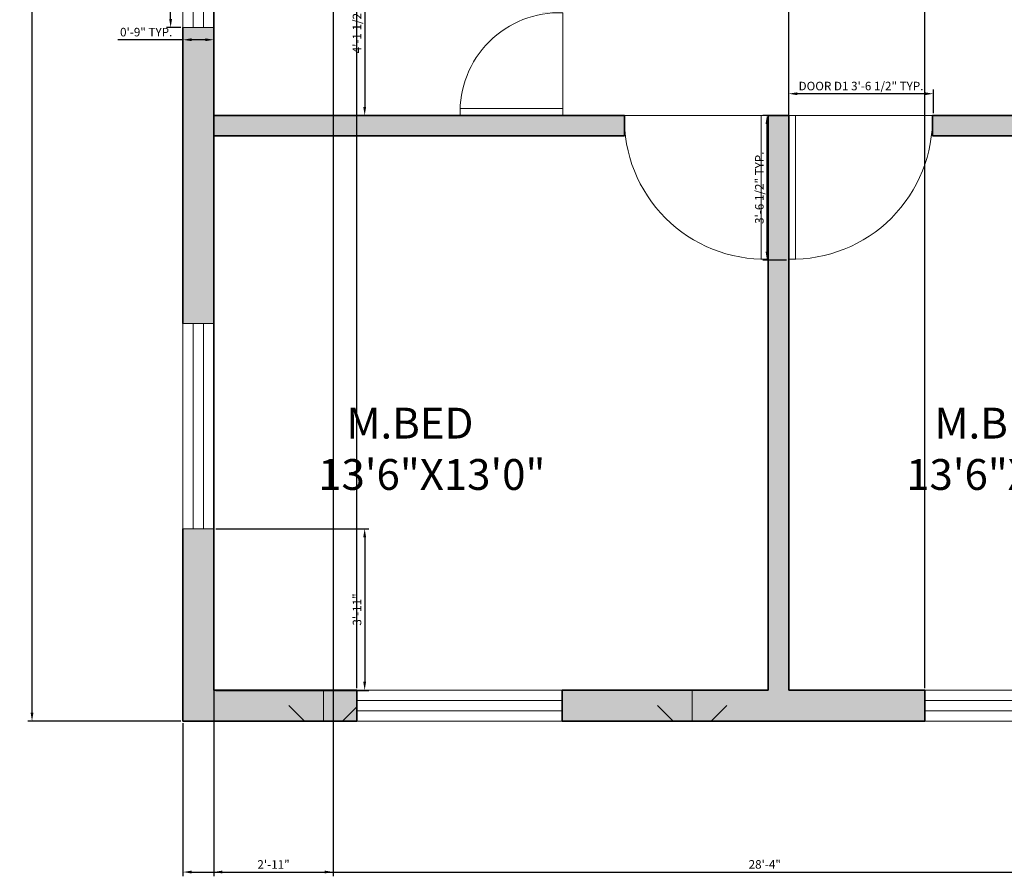
# Model space of a CAD drawing. Units: inches. Extents: x 1851 to 3979, y 3948 to 8145.
# Tile 1 of 4: x 1851 to 2139, y 3948 to 4198. Entities that reach past the tile are written whole.
import ezdxf

# ---------------------------------------------------------------- set-up
doc = ezdxf.new("R2010")
doc.units = ezdxf.units.IN
for name, color, linetype, lineweight in [('A-ANNO-DIMS', 2, 'Continuous', 18), ('A-GLAZ', 140, 'Continuous', 18), ('A-WALL', 7, 'Continuous', 35)]:
    doc.layers.add(name, color=color, linetype=linetype, lineweight=lineweight)
for name, color, linetype, lineweight, true_color in [('A-AREA-IDEN', 9, 'Continuous', 18, 0xc7c8ca), ('A-DOOR', 52, 'Continuous', 18, 0xc8c92d), ('A-WALL-PATT', 159, 'Continuous', 13, 0x22346e)]:
    doc.layers.add(name, color=color, linetype=linetype, lineweight=lineweight, true_color=true_color)
doc.styles.get("Standard").update_dxf_attribs({"font": 'arial.ttf'})
doc.dimstyles.new('ISO-25', dxfattribs={"dimtxt": 2.5, "dimasz": 2.5, "dimexe": 1.25, "dimexo": 0.625, "dimtad": 1, "dimlunit": 3, "dimtxsty": 'Standard', "dimcen": 2.5, "dimadec": 0, "dimazin": 0, "dimtfac": 1, "dimtmove": 0, "dimatfit": 3, "dimfxl": 1, "dimarcsym": 0})

# ---------------------------------------------------------------- blocks, each defined once
blk = doc.blocks.new('DOOR-SINGLE-42IN')
for p, q in [((42, 42), (40, 42)), ((40, 42), (40, 0)), ((42, 0), (42, 42)), ((40, 0), (42, 0))]:
    blk.add_line(p, q)
blk.add_arc((41, 1), 41.01, 88.6028, 181.3972)
blk = doc.blocks.new('DOOR-SINGLE-30IN')
for p, q in [((30, 2), (0, 2)), ((0, 2), (0, 0)), ((0, 0), (30, 0)), ((30, 0), (30, 2))]:
    blk.add_line(p, q)
blk.add_arc((1, 1), 29.02, 358.0251, 91.9749)
blk = doc.blocks.new('WINDOW-60IN')
for p, q in [((0, 9), (60, 9)), ((0, 0), (0, 9)), ((60, 9), (60, 0)), ((0, 6), (60, 6)), ((0, 3), (60, 3)), ((60, 0), (0, 0))]:
    blk.add_line(p, q)
blk = doc.blocks.new('WINDOW-24IN')
for p, q in [((0, 0), (0, 9)), ((0, 9), (24, 9)), ((24, 9), (24, 0)), ((0, 6), (24, 6)), ((0, 3), (24, 3)), ((24, 0), (0, 0))]:
    blk.add_line(p, q)
blk = doc.blocks.new('*D12')
at = {"layer": 'A-ANNO-DIMS', "color": 0, "lineweight": -2, "transparency": 16777216}
for p, q in [((1895.14, 4219.57), (1895.14, 4261.17)), ((1898.11, 4219.57), (1893.89, 4219.57)), ((1895.14, 4198.07), (1895.14, 4217.07)), ((1898.11, 4195.57), (1893.89, 4195.57))]:
    blk.add_line(p, q, dxfattribs=at)
at = {"layer": 'A-ANNO-DIMS', "color": 0, "transparency": 16777216}
for points in [[(1894.72, 4217.07), (1895.55, 4217.07), (1895.14, 4219.57)], [(1894.72, 4198.07), (1895.55, 4198.07), (1895.14, 4195.57)]]:
    blk.add_solid(points, dxfattribs=at)
at = {"layer": 'Defpoints', "color": 0, "transparency": 16777216}
for p in [(1895.14, 4219.57), (1898.74, 4219.57), (1898.74, 4195.57)]:
    blk.add_point(p, dxfattribs=at)
at = {"layer": 'A-ANNO-DIMS', "color": 0, "transparency": 16777216, "insert": (1893.22, 4241.62), "char_height": 2.5, "attachment_point": 5, "rotation": 90}
blk.add_mtext('WINDOW W2 2\'-0" TYP.', dxfattribs=at)
blk = doc.blocks.new('*D13')
at = {"layer": 'A-ANNO-DIMS', "color": 0, "lineweight": -2, "transparency": 16777216}
for p, q in [((1898.74, 4194.95), (1898.74, 4190.72)), ((1907.74, 4194.95), (1907.74, 4190.72)), ((1898.74, 4191.97), (1879.75, 4191.97)), ((1905.24, 4191.97), (1901.24, 4191.97))]:
    blk.add_line(p, q, dxfattribs=at)
at = {"layer": 'A-ANNO-DIMS', "color": 0, "transparency": 16777216}
for points in [[(1901.24, 4192.39), (1901.24, 4191.56), (1898.74, 4191.97)], [(1905.24, 4192.39), (1905.24, 4191.56), (1907.74, 4191.97)]]:
    blk.add_solid(points, dxfattribs=at)
at = {"layer": 'Defpoints', "color": 0, "transparency": 16777216}
for p in [(1898.74, 4195.57), (1907.74, 4195.57), (1898.74, 4191.97)]:
    blk.add_point(p, dxfattribs=at)
at = {"layer": 'A-ANNO-DIMS', "color": 0, "transparency": 16777216, "insert": (1887.99, 4193.88), "char_height": 2.5, "attachment_point": 5}
blk.add_mtext('0\'-9" TYP.', dxfattribs=at)
blk = doc.blocks.new('*D18')
at = {"layer": 'A-ANNO-DIMS', "color": 0, "lineweight": -2, "transparency": 16777216}
for p, q in [((2075.74, 4170.48), (2075.74, 4177.45)), ((2115.51, 4176.2), (2078.24, 4176.2)), ((2118.01, 4170.48), (2118.01, 4177.45))]:
    blk.add_line(p, q, dxfattribs=at)
at = {"layer": 'A-ANNO-DIMS', "color": 0, "transparency": 16777216}
for points in [[(2078.24, 4176.61), (2078.24, 4175.78), (2075.74, 4176.2)], [(2115.51, 4176.61), (2115.51, 4175.78), (2118.01, 4176.2)]]:
    blk.add_solid(points, dxfattribs=at)
at = {"layer": 'Defpoints', "color": 0, "transparency": 16777216}
for p in [(2075.74, 4176.2), (2075.74, 4169.85), (2118.01, 4169.85)]:
    blk.add_point(p, dxfattribs=at)
at = {"layer": 'A-ANNO-DIMS', "color": 0, "transparency": 16777216, "insert": (2096.87, 4178.12), "char_height": 2.5, "attachment_point": 5}
blk.add_mtext('DOOR D1 3\'-6 1/2" TYP.', dxfattribs=at)
blk = doc.blocks.new('*D19')
at = {"layer": 'A-ANNO-DIMS', "color": 0, "lineweight": -2, "transparency": 16777216}
for p, q in [((2075.11, 4169.85), (2068.14, 4169.85)), ((2069.39, 4167.35), (2069.39, 4130.08)), ((2075.11, 4127.58), (2068.14, 4127.58))]:
    blk.add_line(p, q, dxfattribs=at)
at = {"layer": 'A-ANNO-DIMS', "color": 0, "transparency": 16777216}
for points in [[(2068.98, 4167.35), (2069.81, 4167.35), (2069.39, 4169.85)], [(2068.98, 4130.08), (2069.81, 4130.08), (2069.39, 4127.58)]]:
    blk.add_solid(points, dxfattribs=at)
at = {"layer": 'Defpoints', "color": 0, "transparency": 16777216}
for p in [(2075.74, 4169.85), (2069.39, 4127.58), (2075.74, 4127.58)]:
    blk.add_point(p, dxfattribs=at)
at = {"layer": 'A-ANNO-DIMS', "color": 0, "transparency": 16777216, "insert": (2067.48, 4148.72), "char_height": 2.5, "attachment_point": 5, "rotation": 90}
blk.add_mtext('3\'-6 1/2" TYP.', dxfattribs=at)
blk = doc.blocks.new('*D24')
at = {"layer": 'A-ANNO-DIMS', "color": 0, "lineweight": -2, "transparency": 16777216}
for p, q in [((1898.74, 3992.23), (1898.74, 3947.5)), ((2238.74, 3992.23), (2238.74, 3947.5)), ((1901.24, 3948.75), (2236.24, 3948.75))]:
    blk.add_line(p, q, dxfattribs=at)
at = {"layer": 'A-ANNO-DIMS', "color": 0, "transparency": 16777216}
for points in [[(1901.24, 3949.17), (1901.24, 3948.34), (1898.74, 3948.75)], [(2236.24, 3949.17), (2236.24, 3948.34), (2238.74, 3948.75)]]:
    blk.add_solid(points, dxfattribs=at)
at = {"layer": 'Defpoints', "color": 0, "transparency": 16777216}
for p in [(1898.74, 3992.85), (2238.74, 3992.85), (2238.74, 3948.75)]:
    blk.add_point(p, dxfattribs=at)
at = {"layer": 'A-ANNO-DIMS', "color": 0, "transparency": 16777216, "insert": (2068.74, 3950.66), "char_height": 2.5, "attachment_point": 5}
blk.add_mtext('28\'-4"', dxfattribs=at)
blk = doc.blocks.new('*D27')
at = {"layer": 'A-ANNO-DIMS', "color": 0, "lineweight": -2, "transparency": 16777216}
for p, q in [((1907.74, 4002.48), (1907.74, 4473.2)), ((1910.24, 4471.95), (1947.04, 4471.95)), ((1949.54, 4002.48), (1949.54, 4473.2))]:
    blk.add_line(p, q, dxfattribs=at)
at = {"layer": 'A-ANNO-DIMS', "color": 0, "transparency": 16777216}
for points in [[(1910.24, 4472.37), (1910.24, 4471.54), (1907.74, 4471.95)], [(1947.04, 4472.37), (1947.04, 4471.54), (1949.54, 4471.95)]]:
    blk.add_solid(points, dxfattribs=at)
at = {"layer": 'Defpoints', "color": 0, "transparency": 16777216}
for p in [(1949.54, 4471.95), (1907.74, 4001.85), (1949.54, 4001.85)]:
    blk.add_point(p, dxfattribs=at)
at = {"layer": 'A-ANNO-DIMS', "color": 0, "transparency": 16777216, "insert": (1928.64, 4473.86), "char_height": 2.5, "attachment_point": 5}
blk.add_mtext('3\'-6"', dxfattribs=at)
blk = doc.blocks.new('*D28')
at = {"layer": 'A-ANNO-DIMS', "color": 0, "lineweight": -2, "transparency": 16777216}
for p, q in [((2075.74, 4002.48), (2075.74, 4473.2)), ((2078.24, 4471.95), (2113.01, 4471.95)), ((2115.51, 4002.48), (2115.51, 4473.2))]:
    blk.add_line(p, q, dxfattribs=at)
at = {"layer": 'A-ANNO-DIMS', "color": 0, "transparency": 16777216}
for points in [[(2078.24, 4472.37), (2078.24, 4471.54), (2075.74, 4471.95)], [(2113.01, 4472.37), (2113.01, 4471.54), (2115.51, 4471.95)]]:
    blk.add_solid(points, dxfattribs=at)
at = {"layer": 'Defpoints', "color": 0, "transparency": 16777216}
for p in [(2115.51, 4471.95), (2075.74, 4001.85), (2115.51, 4001.85)]:
    blk.add_point(p, dxfattribs=at)
at = {"layer": 'A-ANNO-DIMS', "color": 0, "transparency": 16777216, "insert": (2095.62, 4473.86), "char_height": 2.5, "attachment_point": 5}
blk.add_mtext('3\'-4"', dxfattribs=at)
blk = doc.blocks.new('*D36')
at = {"layer": 'A-ANNO-DIMS', "color": 0, "lineweight": -2, "transparency": 16777216}
for p, q in [((1908.36, 4049.09), (1953.09, 4049.09)), ((1951.84, 4046.59), (1951.84, 4004.35)), ((1908.36, 4001.85), (1953.09, 4001.85))]:
    blk.add_line(p, q, dxfattribs=at)
at = {"layer": 'A-ANNO-DIMS', "color": 0, "transparency": 16777216}
for points in [[(1951.42, 4046.59), (1952.25, 4046.59), (1951.84, 4049.09)], [(1951.42, 4004.35), (1952.25, 4004.35), (1951.84, 4001.85)]]:
    blk.add_solid(points, dxfattribs=at)
at = {"layer": 'Defpoints', "color": 0, "transparency": 16777216}
for p in [(1907.74, 4049.09), (1907.74, 4001.85), (1951.84, 4001.85)]:
    blk.add_point(p, dxfattribs=at)
at = {"layer": 'A-ANNO-DIMS', "color": 0, "transparency": 16777216, "insert": (1949.93, 4025.47), "char_height": 2.5, "attachment_point": 5, "rotation": 90}
blk.add_mtext('3\'-11"', dxfattribs=at)
blk = doc.blocks.new('*D37')
at = {"layer": 'A-ANNO-DIMS', "color": 0, "lineweight": -2, "transparency": 16777216}
for p, q in [((1908.36, 4219.57), (1953.09, 4219.57)), ((1951.84, 4217.07), (1951.84, 4172.35)), ((1908.36, 4169.85), (1953.09, 4169.85))]:
    blk.add_line(p, q, dxfattribs=at)
at = {"layer": 'A-ANNO-DIMS', "color": 0, "transparency": 16777216}
for points in [[(1951.42, 4217.07), (1952.25, 4217.07), (1951.84, 4219.57)], [(1951.42, 4172.35), (1952.25, 4172.35), (1951.84, 4169.85)]]:
    blk.add_solid(points, dxfattribs=at)
at = {"layer": 'Defpoints', "color": 0, "transparency": 16777216}
for p in [(1907.74, 4219.57), (1907.74, 4169.85), (1951.84, 4169.85)]:
    blk.add_point(p, dxfattribs=at)
at = {"layer": 'A-ANNO-DIMS', "color": 0, "transparency": 16777216, "insert": (1949.92, 4194.71), "char_height": 2.5, "attachment_point": 5, "rotation": 90}
blk.add_mtext('4\'-1 1/2"', dxfattribs=at)
blk = doc.blocks.new('*D39')
at = {"layer": 'A-ANNO-DIMS', "color": 0, "lineweight": -2, "transparency": 16777216}
for p, q in [((1927.24, 4427.85), (1853.39, 4427.85)), ((1854.64, 3995.35), (1854.64, 4425.35)), ((1898.11, 3992.85), (1853.39, 3992.85))]:
    blk.add_line(p, q, dxfattribs=at)
at = {"layer": 'A-ANNO-DIMS', "color": 0, "transparency": 16777216}
for points in [[(1854.22, 4425.35), (1855.05, 4425.35), (1854.64, 4427.85)], [(1854.22, 3995.35), (1855.05, 3995.35), (1854.64, 3992.85)]]:
    blk.add_solid(points, dxfattribs=at)
at = {"layer": 'Defpoints', "color": 0, "transparency": 16777216}
for p in [(1854.64, 4427.85), (1927.87, 4427.85), (1898.74, 3992.85)]:
    blk.add_point(p, dxfattribs=at)
at = {"layer": 'A-ANNO-DIMS', "color": 0, "transparency": 16777216, "insert": (1852.73, 4210.35), "char_height": 2.5, "attachment_point": 5, "rotation": 90}
blk.add_mtext('36\'-3"', dxfattribs=at)
blk = doc.blocks.new('*D46')
at = {"layer": 'A-ANNO-DIMS', "color": 0, "lineweight": -2, "transparency": 16777216}
for p, q in [((1907.74, 4403.23), (1907.74, 3947.5)), ((1942.66, 4403.23), (1942.66, 3947.5)), ((1910.24, 3948.75), (1940.16, 3948.75))]:
    blk.add_line(p, q, dxfattribs=at)
at = {"layer": 'A-ANNO-DIMS', "color": 0, "transparency": 16777216}
for points in [[(1910.24, 3949.17), (1910.24, 3948.34), (1907.74, 3948.75)], [(1940.16, 3949.17), (1940.16, 3948.34), (1942.66, 3948.75)]]:
    blk.add_solid(points, dxfattribs=at)
at = {"layer": 'Defpoints', "color": 0, "transparency": 16777216}
for p in [(1907.74, 4403.85), (1942.66, 4403.85), (1942.66, 3948.75)]:
    blk.add_point(p, dxfattribs=at)
at = {"layer": 'A-ANNO-DIMS', "color": 0, "transparency": 16777216, "insert": (1925.2, 3950.64), "char_height": 2.5, "attachment_point": 5}
blk.add_mtext('2\'-11"', dxfattribs=at)

msp = doc.modelspace()

# ---------------------------------------------------------------- hatches: boundary and pattern name
at = {"layer": 'A-WALL-PATT'}
h = msp.add_hatch(dxfattribs=at)
h.set_pattern_fill('GRASS', color=256, scale=3)
h.paths.add_polyline_path([(1942.655, 4412.855), (1898.736, 4412.855), (1898.736, 4348.625), (1907.736, 4348.625), (1907.736, 4403.855), (1942.655, 4403.855)])
h.paths.add_polyline_path([(2027.97, 4412.855), (2002.655, 4412.855), (2002.655, 4403.855), (2027.97, 4403.855, -0.0293864), (2027.97, 4405.855)])
h.paths.add_polyline_path([(2088.59, 4412.855), (2045.97, 4412.855), (2045.97, 4403.855), (2069.736, 4403.855), (2069.736, 4349.855, -0.0172363), (2071.736, 4349.855), (2075.736, 4349.855), (2075.736, 4403.855), (2088.59, 4403.855)])
h.paths.add_polyline_path([(2158.724, 4412.855), (2112.59, 4412.855), (2112.59, 4403.855), (2135.736, 4403.855), (2135.736, 4319.855), (2069.736, 4319.855), (2069.736, 4241.855), (2075.736, 4241.855), (2075.736, 4313.855), (2141.736, 4313.855), (2141.736, 4403.855), (2158.724, 4403.855)])
h.paths.add_polyline_path([(2244.736, 4403.855), (2256.687, 4403.855), (2256.687, 4412.855), (2218.724, 4412.855), (2218.724, 4403.855), (2238.736, 4403.855), (2238.736, 4319.855), (2171.736, 4319.855), (2171.736, 4315.855, -0.0172363), (2171.736, 4313.855), (2238.736, 4313.855), (2238.736, 4211.855), (2242.736, 4211.855, -0.0121933), (2244.736, 4211.855)])
h.paths.add_polyline_path([(2356.912, 4412.855), (2353.884, 4412.855), (2312.372, 4412.855), (2312.372, 4403.855), (2331.736, 4403.855), (2331.736, 4211.855, -0.0121933), (2333.736, 4211.855), (2337.736, 4211.855), (2337.736, 4313.855), (2404.736, 4313.855, -0.0172363), (2404.736, 4315.855), (2404.736, 4319.855), (2337.736, 4319.855), (2337.736, 4403.855), (2353.884, 4403.855), (2356.912, 4403.855)])
h.paths.add_polyline_path([(2440.736, 4403.855), (2451.168, 4403.855), (2451.168, 4412.855), (2401.884, 4412.855), (2401.884, 4403.855), (2434.736, 4403.855), (2434.736, 4313.855), (2500.736, 4313.855), (2500.736, 4241.855), (2506.736, 4241.855), (2506.736, 4283.855), (2506.736, 4319.855), (2476.736, 4319.855), (2440.736, 4319.855)])
h.paths.add_polyline_path([(2506.736, 4403.855), (2516.983, 4403.855), (2516.983, 4412.855), (2475.168, 4412.855), (2475.168, 4403.855), (2500.736, 4403.855), (2500.736, 4349.855), (2504.736, 4349.855, -0.0172363), (2506.736, 4349.855)])
h.paths.add_polyline_path([(2544.739, 4412.855), (2534.983, 4412.855), (2534.983, 4405.855, -0.0293864), (2534.983, 4403.855), (2544.739, 4403.855)])
h.paths.add_polyline_path([(2677.736, 4412.855), (2618.736, 4412.855), (2616.739, 4412.855), (2616.739, 4403.855), (2668.736, 4403.855), (2668.736, 4349.414), (2677.736, 4349.414), (2677.736, 4403.855)])
h.paths.add_polyline_path([(2677.736, 4301.414), (2668.736, 4301.414), (2668.736, 4247.855), (2548.736, 4247.855), (2548.736, 4243.855, -0.0121933), (2548.736, 4241.855), (2572.736, 4241.855), (2572.736, 4187.855, -0.0293864), (2574.736, 4187.855), (2578.736, 4187.855), (2578.736, 4241.855), (2668.736, 4241.855), (2668.736, 4216.247), (2677.736, 4216.247)])
h.paths.add_polyline_path([(2677.736, 4192.247), (2668.736, 4192.247), (2668.736, 4169.855), (2572.736, 4169.855), (2548.736, 4169.855, -0.0424267), (2549.319, 4163.855), (2572.736, 4163.855), (2668.736, 4163.855), (2668.736, 4130.251), (2677.736, 4130.251)])
h.paths.add_polyline_path([(2677.736, 4001.855), (2677.736, 4058.251), (2668.736, 4058.251), (2668.736, 4001.855), (2614.828, 4001.855), (2614.828, 3992.855), (2618.736, 3992.855), (2677.736, 3992.855)])
h.paths.add_polyline_path([(2554.828, 4001.855), (2512.736, 4001.855), (2512.736, 4163.855), (2512.736, 4169.855), (2506.736, 4169.855), (2506.736, 4127.855), (2506.736, 4001.855), (2470.736, 4001.855), (2470.736, 3992.855), (2554.828, 3992.855)])
h.paths.add_polyline_path([(2410.736, 4001.855), (2337.736, 4001.855), (2337.736, 3992.855), (2410.736, 3992.855)])
h.paths.add_polyline_path([(2337.736, 4169.855), (2331.736, 4169.855), (2331.736, 4075.855), (2337.736, 4075.855)])
h.paths.add_polyline_path([(2464.736, 4167.855, -0.0121933), (2464.736, 4169.855), (2337.736, 4169.855), (2337.736, 4163.855), (2464.736, 4163.855)])
h.paths.add_polyline_path([(2244.736, 4169.855), (2202.736, 4169.855), (2117.736, 4169.855, -0.0121933), (2117.736, 4167.855), (2117.736, 4163.855), (2238.736, 4163.855), (2238.736, 4075.855), (2244.736, 4075.855)])
h.paths.add_polyline_path([(2325.736, 4001.855), (2250.736, 4001.855), (2250.736, 3992.855), (2325.736, 3992.855)])
h.paths.add_polyline_path([(2238.736, 4001.855), (2175.511, 4001.855), (2175.511, 3992.855), (2238.736, 3992.855)])
h.paths.add_polyline_path([(2115.511, 4001.855), (2075.736, 4001.855), (2075.736, 4169.855), (2069.736, 4169.855), (2069.736, 4127.855), (2069.736, 4001.855), (2009.539, 4001.855), (2009.539, 3992.855), (2115.511, 3992.855)])
h.paths.add_polyline_path([(1949.539, 4001.855), (1907.736, 4001.855), (1907.736, 4049.088), (1898.736, 4049.088), (1898.736, 3992.855), (1949.539, 3992.855)])
h.paths.add_polyline_path([(1907.736, 4163.855), (2027.736, 4163.855), (2027.736, 4167.855, -0.0121933), (2027.736, 4169.855), (1907.736, 4169.855), (1907.736, 4195.575), (1898.736, 4195.575), (1898.736, 4109.088), (1907.736, 4109.088)])
h.paths.add_polyline_path([(2027.736, 4247.855), (1907.736, 4247.855), (1907.736, 4288.625), (1898.736, 4288.625), (1898.736, 4219.575), (1907.736, 4219.575), (1907.736, 4241.855), (2003.736, 4241.855), (2003.736, 4219.575), (2003.736, 4199.855), (2007.736, 4199.855, -0.0172363), (2009.736, 4199.855), (2009.736, 4241.855), (2027.736, 4241.855, -0.0121933), (2027.736, 4243.855)])
h = msp.add_hatch(dxfattribs=at)
h.set_pattern_fill('GRASS', color=256, scale=3)
h.paths.add_polyline_path([(1907.736, 4403.855), (1942.655, 4403.855), (1942.655, 4412.855), (1898.736, 4412.855), (1898.736, 4348.625), (1907.736, 4348.625)])
h.paths.add_polyline_path([(1907.736, 4288.625), (1898.736, 4288.625), (1898.736, 4219.575), (1907.736, 4219.575), (1907.736, 4241.855), (2003.736, 4241.855), (2003.736, 4219.575), (2003.736, 4199.855), (2007.736, 4199.855, -0.0172363), (2009.736, 4199.855), (2009.736, 4241.855), (2027.736, 4241.855, -0.0121933), (2027.736, 4243.855), (2027.736, 4247.855), (1907.736, 4247.855)])
h.paths.add_polyline_path([(1907.736, 4163.855), (2027.736, 4163.855), (2027.736, 4167.855, -0.0121933), (2027.736, 4169.855), (1907.736, 4169.855), (1907.736, 4195.575), (1898.736, 4195.575), (1898.736, 4109.088), (1907.736, 4109.088)])
h.paths.add_polyline_path([(1907.736, 4049.088), (1898.736, 4049.088), (1898.736, 3992.855), (1949.539, 3992.855), (1949.539, 4001.855), (1907.736, 4001.855)])
h = msp.add_hatch(color=256, dxfattribs=at)
h.dxf.hatch_style = 1
h.paths.add_polyline_path([(1907.736, 4163.855), (2027.736, 4163.855), (2027.736, 4167.855, -0.0121933), (2027.736, 4169.855), (1907.736, 4169.855), (1907.736, 4195.575), (1898.736, 4195.575), (1898.736, 4109.088), (1907.736, 4109.088)])
h.paths.add_polyline_path([(1907.736, 4049.088), (1898.736, 4049.088), (1898.736, 3992.855), (1949.539, 3992.855), (1949.539, 4001.855), (1907.736, 4001.855)])
h.paths.add_polyline_path([(2115.511, 4001.855), (2075.736, 4001.855), (2075.736, 4169.855), (2069.736, 4169.855), (2069.736, 4127.855), (2069.736, 4001.855), (2009.539, 4001.855), (2009.539, 3992.855), (2115.511, 3992.855)])
h.paths.add_polyline_path([(2238.736, 4001.855), (2175.511, 4001.855), (2175.511, 3992.855), (2238.736, 3992.855)])
h.paths.add_polyline_path([(2325.736, 4001.855), (2250.736, 4001.855), (2250.736, 3992.855), (2325.736, 3992.855)])
h.paths.add_polyline_path([(2410.736, 4001.855), (2337.736, 4001.855), (2337.736, 3992.855), (2410.736, 3992.855)])
h.paths.add_polyline_path([(2554.828, 4001.855), (2512.736, 4001.855), (2512.736, 4163.855), (2512.736, 4169.855), (2506.736, 4169.855), (2506.736, 4127.855), (2506.736, 4001.855), (2470.736, 4001.855), (2470.736, 3992.855), (2554.828, 3992.855)])
h.paths.add_polyline_path([(2677.736, 4001.855), (2677.736, 4058.251), (2668.736, 4058.251), (2668.736, 4001.855), (2614.828, 4001.855), (2614.828, 3992.855), (2618.736, 3992.855), (2677.736, 3992.855)])
h.paths.add_polyline_path([(2244.736, 4169.855), (2202.736, 4169.855), (2117.736, 4169.855, -0.0121933), (2117.736, 4167.855), (2117.736, 4163.855), (2238.736, 4163.855), (2238.736, 4075.855), (2244.736, 4075.855)])
h.paths.add_polyline_path([(2337.736, 4169.855), (2331.736, 4169.855), (2331.736, 4075.855), (2337.736, 4075.855)])
h.paths.add_polyline_path([(2337.736, 4063.855), (2331.736, 4063.855), (2331.736, 4004.855), (2337.736, 4004.855)])
h.paths.add_polyline_path([(2244.736, 4063.855), (2238.736, 4063.855), (2238.736, 4004.855), (2244.736, 4004.855)])
h.paths.add_polyline_path([(2464.736, 4167.855, -0.0121933), (2464.736, 4169.855), (2337.736, 4169.855), (2337.736, 4163.855), (2464.736, 4163.855)])
h.paths.add_polyline_path([(2337.736, 4313.855), (2404.736, 4313.855, -0.0172363), (2404.736, 4315.855), (2404.736, 4319.855), (2337.736, 4319.855), (2337.736, 4403.855), (2353.884, 4403.855), (2356.912, 4403.855), (2356.912, 4412.855), (2353.884, 4412.855), (2312.372, 4412.855), (2312.372, 4403.855), (2331.736, 4403.855), (2331.736, 4211.855, -0.0121933), (2333.736, 4211.855), (2337.736, 4211.855)])
h.paths.add_polyline_path([(2244.736, 4403.855), (2256.687, 4403.855), (2256.687, 4412.855), (2218.724, 4412.855), (2218.724, 4403.855), (2238.736, 4403.855), (2238.736, 4319.855), (2171.736, 4319.855), (2171.736, 4315.855, -0.0172363), (2171.736, 4313.855), (2238.736, 4313.855), (2238.736, 4211.855), (2242.736, 4211.855, -0.0121933), (2244.736, 4211.855)])
h.paths.add_polyline_path([(2506.736, 4283.855), (2506.736, 4319.855), (2476.736, 4319.855), (2440.736, 4319.855), (2440.736, 4403.855), (2451.168, 4403.855), (2451.168, 4412.855), (2401.884, 4412.855), (2401.884, 4403.855), (2434.736, 4403.855), (2434.736, 4313.855), (2500.736, 4313.855), (2500.736, 4241.855), (2506.736, 4241.855)])
h.paths.add_polyline_path([(2578.736, 4241.855), (2668.736, 4241.855), (2668.736, 4216.247), (2677.736, 4216.247), (2677.736, 4301.414), (2668.736, 4301.414), (2668.736, 4247.855), (2548.736, 4247.855), (2548.736, 4243.855, -0.0121933), (2548.736, 4241.855), (2572.736, 4241.855), (2572.736, 4187.855, -0.0293864), (2574.736, 4187.855), (2578.736, 4187.855)])
h.paths.add_polyline_path([(2677.736, 4192.247), (2668.736, 4192.247), (2668.736, 4169.855), (2572.736, 4169.855), (2548.736, 4169.855, -0.0424267), (2549.319, 4163.855), (2572.736, 4163.855), (2668.736, 4163.855), (2668.736, 4130.251), (2677.736, 4130.251)])
h.paths.add_polyline_path([(2506.736, 4403.855), (2516.983, 4403.855), (2516.983, 4412.855), (2475.168, 4412.855), (2475.168, 4403.855), (2500.736, 4403.855), (2500.736, 4349.855), (2504.736, 4349.855, -0.0172363), (2506.736, 4349.855)])
h.paths.add_polyline_path([(2677.736, 4412.855), (2618.736, 4412.855), (2616.739, 4412.855), (2616.739, 4403.855), (2668.736, 4403.855), (2668.736, 4349.414), (2677.736, 4349.414), (2677.736, 4403.855)])
h.paths.add_polyline_path([(2544.739, 4412.855), (2534.983, 4412.855), (2534.983, 4405.855, -0.0293864), (2534.983, 4403.855), (2544.739, 4403.855)])
h.paths.add_polyline_path([(2141.736, 4403.855), (2158.724, 4403.855), (2158.724, 4412.855), (2112.59, 4412.855), (2112.59, 4403.855), (2135.736, 4403.855), (2135.736, 4319.855), (2069.736, 4319.855), (2069.736, 4241.855), (2075.736, 4241.855), (2075.736, 4313.855), (2141.736, 4313.855), (2141.736, 4343.855)])
h.paths.add_polyline_path([(2075.736, 4403.855), (2088.59, 4403.855), (2088.59, 4412.855), (2045.97, 4412.855), (2045.97, 4403.855), (2069.736, 4403.855), (2069.736, 4349.855, -0.0172363), (2071.736, 4349.855), (2075.736, 4349.855)])
h.paths.add_polyline_path([(2027.97, 4412.855), (2002.655, 4412.855), (2002.655, 4403.855), (2027.97, 4403.855, -0.0293864), (2027.97, 4405.855)])
h.paths.add_polyline_path([(1942.655, 4412.855), (1898.736, 4412.855), (1898.736, 4348.625), (1907.736, 4348.625), (1907.736, 4403.855), (1942.655, 4403.855)])
h.paths.add_polyline_path([(2027.736, 4247.855), (1907.736, 4247.855), (1907.736, 4288.625), (1898.736, 4288.625), (1898.736, 4219.575), (1907.736, 4219.575), (1907.736, 4241.855), (2003.736, 4241.855), (2003.736, 4219.575), (2003.736, 4199.855), (2007.736, 4199.855, -0.0172363), (2009.736, 4199.855), (2009.736, 4241.855), (2027.736, 4241.855, -0.0121933), (2027.736, 4243.855)])

# ---------------------------------------------------------------- linework, layer by layer
at = {"layer": 'A-DOOR'}
for p, q in [((2009.736, 4170.855), (2009.736, 4199.855)), ((2027.736, 4169.855), (2068.736, 4169.855)), ((2075.736, 4169.855), (2117.736, 4169.855))]:
    msp.add_line(p, q, dxfattribs=at)
at = {"layer": 'A-GLAZ'}
for p, q in [((1898.736, 4195.575), (1907.736, 4195.575)), ((1898.736, 4109.088), (1907.736, 4109.088)), ((1898.736, 4049.088), (1907.736, 4049.088))]:
    msp.add_line(p, q, dxfattribs=at)
at = {"layer": 'A-WALL'}
for p, q in [((1898.736, 4109.088), (1898.736, 4195.575)), ((1907.736, 4169.855), (1907.736, 4195.575)), ((2027.736, 4169.855), (1907.736, 4169.855)), ((2027.736, 4169.855), (2027.736, 4163.855)), ((2069.736, 4169.855), (2069.736, 4001.855)), ((2075.736, 4169.855), (2069.736, 4169.855)), ((2075.736, 4169.855), (2075.736, 4001.855)), ((2244.736, 4169.855), (2117.736, 4169.855)), ((2117.736, 4169.855), (2117.736, 4163.855)), ((2027.736, 4163.855), (1907.736, 4163.855)), ((1907.736, 4109.088), (1907.736, 4163.855)), ((2238.736, 4163.855), (2117.736, 4163.855)), ((1898.736, 3992.855), (1898.736, 4049.088)), ((1907.736, 4001.855), (1907.736, 4049.088)), ((1949.539, 4001.855), (1907.736, 4001.855)), ((1949.539, 4001.855), (1949.539, 3992.855)), ((2069.736, 4001.855), (2009.539, 4001.855)), ((2009.539, 4001.855), (2009.539, 3992.855)), ((2115.511, 4001.855), (2075.736, 4001.855)), ((2115.511, 4001.855), (2115.511, 3992.855)), ((1949.539, 3992.855), (1898.736, 3992.855)), ((2115.511, 3992.855), (2009.539, 3992.855))]:
    msp.add_line(p, q, dxfattribs=at)

# ---------------------------------------------------------------- block references
at = {"layer": 'A-DOOR', "extrusion": (0, 0, -1), "zscale": -1}
msp.add_blockref('DOOR-SINGLE-30IN', (-2009.736, 4169.855), dxfattribs=at)
at = {"layer": 'A-DOOR', "extrusion": (0, 0, -1), "zscale": -1, "rotation": 180}
msp.add_blockref('DOOR-SINGLE-42IN', (-2027.736, 4169.855), dxfattribs=at)
at = {"layer": 'A-DOOR', "rotation": 180}
msp.add_blockref('DOOR-SINGLE-42IN', (2117.736, 4169.855), dxfattribs=at)
at = {"layer": 'A-GLAZ'}
for name, p, rotation in [('WINDOW-24IN', (1907.736, 4195.575), 89.9999999999931), ('WINDOW-60IN', (1898.736, 4109.088), 270.0000000000025), ('WINDOW-60IN', (2009.539, 4001.855), 180), ('WINDOW-60IN', (2175.511, 4001.855), 180)]:
    msp.add_blockref(name, p, dxfattribs=dict(at, rotation=rotation))

# ---------------------------------------------------------------- texts
at = {"layer": 'A-AREA-IDEN', "char_height": 9, "attachment_point": 1}
for insert in [(1938.246, 4084.435), (2110.069, 4084.435)]:
    msp.add_mtext_dynamic_manual_height_columns('  { M.BED \\P13\'6"X13\'0"}', width=73.08431, gutter_width=12.5, heights=[0], dxfattribs=dict(at, insert=insert))

# ---------------------------------------------------------------- dimensions: what is measured, and where the dimension line sits
at = {"layer": 'A-ANNO-DIMS'}
for base, p1, p2, picture, middle in [((1949.539, 4471.955), (1907.736, 4001.855), (1949.539, 4001.855), '*D27', (1928.638, 4473.857)), ((2115.511, 4471.955), (2075.736, 4001.855), (2115.511, 4001.855), '*D28', (2095.623, 4473.857)), ((1942.655, 3948.755), (1907.736, 4403.855), (1942.655, 4403.855), '*D46', (1925.196, 3950.635)), ((2238.736, 3948.755), (1898.736, 3992.855), (2238.736, 3992.855), '*D24', (2068.736, 3950.656))]:
    dim = msp.add_linear_dim(base=base, p1=p1, p2=p2, dimstyle='ISO-25', override={"dimdec": 1, "dimlfac": 1, "dimrnd": 0, "dimzin": 1, "dimdsep": 46, "dimlunit": 4, "dimfrac": 2}, dxfattribs=at)
    dim.commit()
    dim.dimension.update_dxf_attribs({"geometry": picture, "text_midpoint": middle})
for base, p1, p2, angle, picture, middle in [((1854.636, 4427.855), (1898.736, 3992.855), (1927.869, 4427.855), 90, '*D39', (1852.734, 4210.355)), ((1951.836, 4169.855), (1907.736, 4219.575), (1907.736, 4169.855), 270, '*D37', (1949.918, 4194.715)), ((1951.836, 4001.855), (1907.736, 4049.088), (1907.736, 4001.855), 270, '*D36', (1949.934, 4025.471))]:
    dim = msp.add_linear_dim(base=base, p1=p1, p2=p2, angle=angle, dimstyle='ISO-25', override={"dimdec": 1, "dimlfac": 1, "dimrnd": 0, "dimzin": 1, "dimdsep": 46, "dimlunit": 4, "dimfrac": 2}, dxfattribs=at)
    dim.commit()
    dim.dimension.update_dxf_attribs({"geometry": picture, "text_midpoint": middle})
for base, p1, p2, angle, text, picture, middle in [((1895.136, 4219.575), (1898.736, 4195.575), (1898.736, 4219.575), 90, 'WINDOW W2 <> TYP.', '*D12', (1893.218, 4241.622)), ((1898.736, 4191.975), (1907.736, 4195.575), (1898.736, 4195.575), 180, '<> TYP.', '*D13', (1887.992, 4193.876)), ((2075.736, 4176.196), (2118.01, 4169.855), (2075.736, 4169.855), 180, 'DOOR D1 <> TYP.', '*D18', (2096.873, 4178.115)), ((2069.395, 4127.581), (2075.736, 4169.855), (2075.736, 4127.581), 270, '<> TYP.', '*D19', (2067.476, 4148.718))]:
    dim = msp.add_linear_dim(base=base, p1=p1, p2=p2, angle=angle, text=text, dimstyle='ISO-25', override={"dimdec": 1, "dimlfac": 1, "dimrnd": 0, "dimzin": 1, "dimdsep": 46, "dimlunit": 4, "dimfrac": 2}, dxfattribs=at)
    dim.commit()
    dim.dimension.update_dxf_attribs({"geometry": picture, "text_midpoint": middle})

doc.saveas('drawing.dxf')
